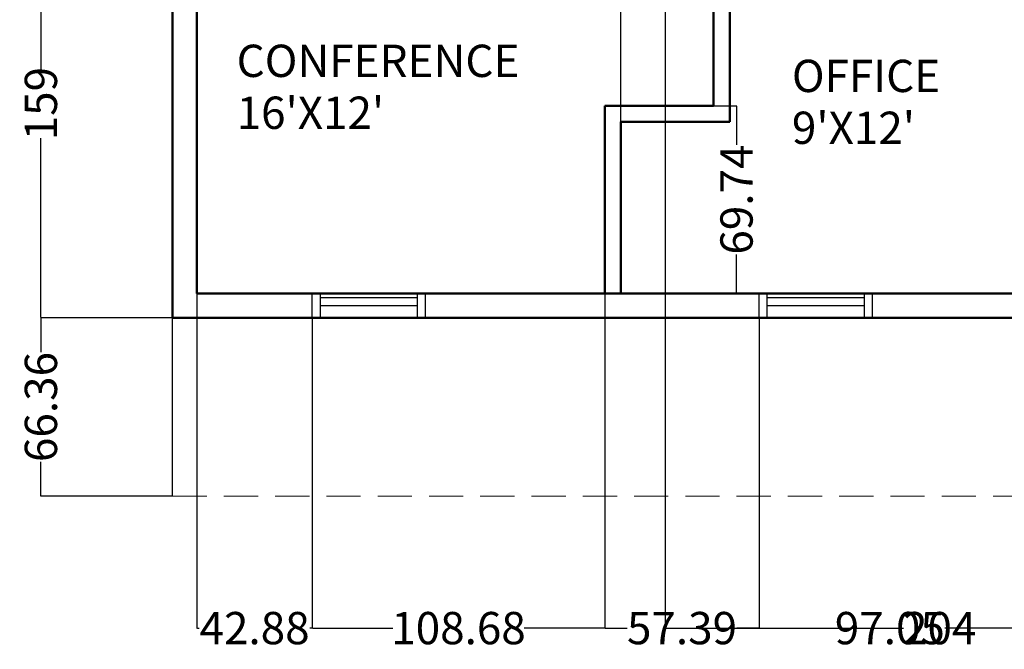
# Model space of a CAD drawing. Units: inches. Extents: x 128 to 1267, y -109 to 1208.
# Tile 5 of 8: x 180 to 546, y 608 to 842. Entities that reach past the tile are written whole.
import ezdxf

# ---------------------------------------------------------------- set-up
doc = ezdxf.new("R2010")
doc.units = ezdxf.units.IN
doc.header["$MEASUREMENT"] = 0
doc.linetypes.add('DASHED', pattern=[19.05, 12.7, -6.35])
for name, color, linetype, lineweight in [('A-ANNO-DIMS', 2, 'Continuous', 18), ('A-AREA-IDEN', 3, 'Continuous', 25), ('A-GLAZ', 3, 'Continuous', 25), ('A-ROOF-OVHD', 9, 'DASHED', 18), ('A-WALL', 7, 'Continuous', 50)]:
    doc.layers.add(name, color=color, linetype=linetype, lineweight=lineweight)
doc.styles.get("Standard").update_dxf_attribs({"font": 'arial.ttf'})
doc.dimstyles.get("Standard").update_dxf_attribs({"dimtxt": 12, "dimasz": 0.18, "dimexe": 0.18, "dimexo": 0.0625, "dimgap": 0.09, "dimtad": 0, "dimdec": 1, "dimzin": 0, "dimdsep": 46, "dimlunit": 3, "dimtxsty": 'Standard', "dimcen": 0.09, "dimadec": 0, "dimazin": 0, "dimtfac": 1, "dimtdec": 1, "dimtofl": 0, "dimtmove": 0, "dimatfit": 3, "dimfxl": 1, "dimtolj": 1, "dimtzin": 0, "dimarcsym": 0})

# ---------------------------------------------------------------- blocks, each defined once
blk = doc.blocks.new('WIN-900')
for p, q in [((1102.06, 345.56), (1111.06, 345.56)), ((1102.06, 342.56), (1111.06, 342.56)), ((1103.56, 306.56), (1103.56, 342.56)), ((1106.56, 306.56), (1106.56, 342.56)), ((1111.06, 306.56), (1102.06, 306.56)), ((1111.06, 303.56), (1102.06, 303.56))]:
    blk.add_line(p, q)
blk = doc.blocks.new('*D93')
at = {"layer": 'A-ANNO-DIMS', "color": 0, "lineweight": -2, "transparency": 16777216}
for p, q in [((237.13, 664.93), (237.13, 1188.36)), ((237.31, 1188.18), (667.76, 1188.18)), ((1124.95, 1188.18), (694.49, 1188.18)), ((1125.13, 664.93), (1125.13, 1188.36))]:
    blk.add_line(p, q, dxfattribs=at)
at = {"layer": 'A-ANNO-DIMS', "color": 0, "transparency": 16777216}
for points in [[(237.31, 1188.21), (237.31, 1188.15), (237.13, 1188.18)], [(1124.95, 1188.21), (1124.95, 1188.15), (1125.13, 1188.18)]]:
    blk.add_solid(points, dxfattribs=at)
at = {"layer": 'Defpoints', "color": 0, "transparency": 16777216}
for p in [(1125.13, 1188.18), (237.13, 664.87), (1125.13, 664.87)]:
    blk.add_point(p, dxfattribs=at)
at = {"layer": 'A-ANNO-DIMS', "color": 0, "transparency": 16777216, "insert": (681.13, 1188.18), "char_height": 12, "attachment_point": 5}
blk.add_mtext('\\A1;888', dxfattribs=at)
blk = doc.blocks.new('*D96')
at = {"layer": 'A-ANNO-DIMS', "color": 0, "lineweight": -2, "transparency": 16777216}
for p, q in [((237.06, 731.23), (188, 731.23)), ((188.18, 731.05), (188.18, 718.41)), ((188.18, 665.05), (188.18, 677.68)), ((237.06, 664.87), (188, 664.87))]:
    blk.add_line(p, q, dxfattribs=at)
at = {"layer": 'A-ANNO-DIMS', "color": 0, "transparency": 16777216}
for points in [[(188.15, 731.05), (188.21, 731.05), (188.18, 731.23)], [(188.15, 665.05), (188.21, 665.05), (188.18, 664.87)]]:
    blk.add_solid(points, dxfattribs=at)
at = {"layer": 'Defpoints', "color": 0, "transparency": 16777216}
for p in [(237.13, 731.23), (188.18, 664.87), (237.13, 664.87)]:
    blk.add_point(p, dxfattribs=at)
at = {"layer": 'A-ANNO-DIMS', "color": 0, "transparency": 16777216, "insert": (188.18, 698.05), "char_height": 12, "attachment_point": 5, "rotation": 90}
blk.add_mtext('\\A1;66.36', dxfattribs=at)
blk = doc.blocks.new('*D112')
at = {"layer": 'A-ANNO-DIMS', "color": 0, "lineweight": -2, "transparency": 16777216}
for p, q in [((246.13, 740.16), (246.13, 615.74)), ((289.01, 731.16), (289.01, 615.74)), ((246.31, 615.92), (246.98, 615.92)), ((288.83, 615.92), (288.16, 615.92))]:
    blk.add_line(p, q, dxfattribs=at)
at = {"layer": 'A-ANNO-DIMS', "color": 0, "transparency": 16777216}
for points in [[(246.31, 615.95), (246.31, 615.89), (246.13, 615.92)], [(288.83, 615.95), (288.83, 615.89), (289.01, 615.92)]]:
    blk.add_solid(points, dxfattribs=at)
at = {"layer": 'Defpoints', "color": 0, "transparency": 16777216}
for p in [(246.13, 740.23), (289.01, 731.23), (289.01, 615.92)]:
    blk.add_point(p, dxfattribs=at)
at = {"layer": 'A-ANNO-DIMS', "color": 0, "transparency": 16777216, "insert": (267.57, 615.92), "char_height": 12, "attachment_point": 5}
blk.add_mtext('\\A1;42.88', dxfattribs=at)
blk = doc.blocks.new('*D113')
at = {"layer": 'A-ANNO-DIMS', "color": 0, "lineweight": -2, "transparency": 16777216}
for p, q in [((397.68, 740.16), (397.68, 615.74)), ((289.01, 731.16), (289.01, 615.74)), ((289.19, 615.92), (318.9, 615.92)), ((397.5, 615.92), (367.79, 615.92))]:
    blk.add_line(p, q, dxfattribs=at)
at = {"layer": 'A-ANNO-DIMS', "color": 0, "transparency": 16777216}
for points in [[(289.19, 615.95), (289.19, 615.89), (289.01, 615.92)], [(397.5, 615.95), (397.5, 615.89), (397.68, 615.92)]]:
    blk.add_solid(points, dxfattribs=at)
at = {"layer": 'Defpoints', "color": 0, "transparency": 16777216}
for p in [(397.68, 740.23), (289.01, 731.23), (397.68, 615.92)]:
    blk.add_point(p, dxfattribs=at)
at = {"layer": 'A-ANNO-DIMS', "color": 0, "transparency": 16777216, "insert": (343.34, 615.92), "char_height": 12, "attachment_point": 5}
blk.add_mtext('\\A1;108.68', dxfattribs=at)
blk = doc.blocks.new('*D114')
at = {"layer": 'A-ANNO-DIMS', "color": 0, "lineweight": -2, "transparency": 16777216}
for p, q in [((397.68, 740.16), (397.68, 615.74)), ((455.08, 731.16), (455.08, 615.74)), ((397.86, 615.92), (406.03, 615.92)), ((454.9, 615.92), (446.73, 615.92))]:
    blk.add_line(p, q, dxfattribs=at)
at = {"layer": 'A-ANNO-DIMS', "color": 0, "transparency": 16777216}
for points in [[(397.86, 615.95), (397.86, 615.89), (397.68, 615.92)], [(454.9, 615.95), (454.9, 615.89), (455.08, 615.92)]]:
    blk.add_solid(points, dxfattribs=at)
at = {"layer": 'Defpoints', "color": 0, "transparency": 16777216}
for p in [(397.68, 740.23), (455.08, 731.23), (455.08, 615.92)]:
    blk.add_point(p, dxfattribs=at)
at = {"layer": 'A-ANNO-DIMS', "color": 0, "transparency": 16777216, "insert": (426.38, 615.92), "char_height": 12, "attachment_point": 5}
blk.add_mtext('\\A1;57.39', dxfattribs=at)
blk = doc.blocks.new('*D115')
at = {"layer": 'A-ANNO-DIMS', "color": 0, "lineweight": -2, "transparency": 16777216}
for p, q in [((552.13, 740.16), (552.13, 615.74)), ((455.08, 731.16), (455.08, 615.74)), ((455.26, 615.92), (483.22, 615.92)), ((551.95, 615.92), (523.98, 615.92))]:
    blk.add_line(p, q, dxfattribs=at)
at = {"layer": 'A-ANNO-DIMS', "color": 0, "transparency": 16777216}
for points in [[(455.26, 615.95), (455.26, 615.89), (455.08, 615.92)], [(551.95, 615.95), (551.95, 615.89), (552.13, 615.92)]]:
    blk.add_solid(points, dxfattribs=at)
at = {"layer": 'Defpoints', "color": 0, "transparency": 16777216}
for p in [(552.13, 740.23), (455.08, 731.23), (552.13, 615.92)]:
    blk.add_point(p, dxfattribs=at)
at = {"layer": 'A-ANNO-DIMS', "color": 0, "transparency": 16777216, "insert": (503.6, 615.92), "char_height": 12, "attachment_point": 5}
blk.add_mtext('\\A1;97.05', dxfattribs=at)
blk = doc.blocks.new('*D126')
at = {"layer": 'A-ANNO-DIMS', "color": 0, "lineweight": -2, "transparency": 16777216}
for p, q in [((246.06, 890.23), (188, 890.23)), ((188.18, 890.05), (188.18, 823.52)), ((188.18, 731.41), (188.18, 797.93)), ((237.06, 731.23), (188, 731.23))]:
    blk.add_line(p, q, dxfattribs=at)
at = {"layer": 'A-ANNO-DIMS', "color": 0, "transparency": 16777216}
for points in [[(188.15, 890.05), (188.21, 890.05), (188.18, 890.23)], [(188.15, 731.41), (188.21, 731.41), (188.18, 731.23)]]:
    blk.add_solid(points, dxfattribs=at)
at = {"layer": 'Defpoints', "color": 0, "transparency": 16777216}
for p in [(188.18, 890.23), (246.13, 890.23), (237.13, 731.23)]:
    blk.add_point(p, dxfattribs=at)
at = {"layer": 'A-ANNO-DIMS', "color": 0, "transparency": 16777216, "insert": (188.18, 810.73), "char_height": 12, "attachment_point": 5, "rotation": 90}
blk.add_mtext('\\A1;159', dxfattribs=at)
blk = doc.blocks.new('*D140')
at = {"layer": 'A-ANNO-DIMS', "color": 0, "lineweight": -2, "transparency": 16777216}
for p, q in [((397.74, 809.97), (446.81, 809.97)), ((446.63, 809.79), (446.63, 795.44)), ((446.63, 740.41), (446.63, 754.75)), ((397.74, 740.23), (446.81, 740.23))]:
    blk.add_line(p, q, dxfattribs=at)
at = {"layer": 'A-ANNO-DIMS', "color": 0, "transparency": 16777216}
for points in [[(446.6, 809.79), (446.66, 809.79), (446.63, 809.97)], [(446.6, 740.41), (446.66, 740.41), (446.63, 740.23)]]:
    blk.add_solid(points, dxfattribs=at)
at = {"layer": 'Defpoints', "color": 0, "transparency": 16777216}
for p in [(397.68, 809.97), (397.68, 740.23), (446.63, 740.23)]:
    blk.add_point(p, dxfattribs=at)
at = {"layer": 'A-ANNO-DIMS', "color": 0, "transparency": 16777216, "insert": (446.63, 775.1), "char_height": 12, "attachment_point": 5, "rotation": 90}
blk.add_mtext('\\A1;69.74', dxfattribs=at)
blk = doc.blocks.new('*D141')
at = {"layer": 'A-ANNO-DIMS', "color": 0, "lineweight": -2, "transparency": 16777216}
for p, q in [((403.68, 804.03), (403.68, 853.1)), ((403.86, 852.92), (443.95, 852.92)), ((444.13, 804.03), (444.13, 853.1)), ((444.13, 852.92), (444.31, 852.92))]:
    blk.add_line(p, q, dxfattribs=at)
at = {"layer": 'A-ANNO-DIMS', "color": 0, "transparency": 16777216}
for points in [[(403.86, 852.95), (403.86, 852.89), (403.68, 852.92)], [(443.95, 852.95), (443.95, 852.89), (444.13, 852.92)]]:
    blk.add_solid(points, dxfattribs=at)
at = {"layer": 'Defpoints', "color": 0, "transparency": 16777216}
for p in [(444.13, 852.92), (403.68, 803.97), (444.13, 803.97)]:
    blk.add_point(p, dxfattribs=at)
at = {"layer": 'A-ANNO-DIMS', "color": 0, "transparency": 16777216, "insert": (469.59, 852.92), "char_height": 12, "attachment_point": 5}
blk.add_mtext('\\A1;40.445', dxfattribs=at)
blk = doc.blocks.new('*D148')
at = {"layer": 'A-ANNO-DIMS', "color": 0, "lineweight": -2, "transparency": 16777216}
for p, q in [((420.13, 968.16), (420.13, 615.74)), ((624.13, 968.16), (624.13, 615.74)), ((420.31, 615.92), (508.7, 615.92)), ((623.95, 615.92), (535.55, 615.92))]:
    blk.add_line(p, q, dxfattribs=at)
at = {"layer": 'A-ANNO-DIMS', "color": 0, "transparency": 16777216}
for points in [[(420.31, 615.95), (420.31, 615.89), (420.13, 615.92)], [(623.95, 615.95), (623.95, 615.89), (624.13, 615.92)]]:
    blk.add_solid(points, dxfattribs=at)
at = {"layer": 'Defpoints', "color": 0, "transparency": 16777216}
for p in [(420.13, 968.23), (624.13, 968.23), (624.13, 615.92)]:
    blk.add_point(p, dxfattribs=at)
at = {"layer": 'A-ANNO-DIMS', "color": 0, "transparency": 16777216, "insert": (522.13, 615.92), "char_height": 12, "attachment_point": 5}
blk.add_mtext('\\A1;204', dxfattribs=at)

msp = doc.modelspace()

# ---------------------------------------------------------------- linework, layer by layer
at = {"layer": 'A-ROOF-OVHD'}
for p, q in [((237.1268, 731.2265), (237.1268, 664.8687)), ((237.1268, 664.8687), (1125.1268, 664.8687))]:
    msp.add_line(p, q, dxfattribs=at)
at = {"layer": 'A-WALL'}
for p, q in [((246.1268, 884.2265), (246.1268, 740.2265)), ((438.1268, 884.2265), (438.1268, 809.9714)), ((444.1268, 884.2265), (444.1268, 803.9714)), ((438.1268, 809.9714), (397.6821, 809.9714)), ((397.6821, 809.9714), (397.6821, 740.2265)), ((438.1268, 803.9714), (403.6821, 803.9714)), ((403.6821, 803.9714), (403.6821, 740.2265)), ((444.1268, 803.9714), (438.1268, 803.9714)), ((246.1268, 740.2265), (552.1268, 740.2265)), ((444.1268, 740.2265), (552.1268, 740.2265)), ((444.1268, 740.2265), (552.1268, 740.2265))]:
    msp.add_line(p, q, dxfattribs=at)
msp.add_lwpolyline([(1110.1268, 731.2265), (1125.1268, 731.2265), (1125.1268, 1139.2265), (237.1268, 1139.2265), (237.1268, 731.2265), (1038.1268, 731.2265)], dxfattribs=at)

# ---------------------------------------------------------------- block references
at = {"layer": 'A-GLAZ'}
for p, rotation in [((-14.5573, 1842.2825), 270.0000000000003), ((151.514, 1842.2825), 270.0000000000002)]:
    msp.add_blockref('WIN-900', p, dxfattribs=dict(at, rotation=rotation))

# ---------------------------------------------------------------- texts
at = {"layer": 'A-AREA-IDEN'}
for s, p in [('CONFERENCE', (260.9026, 820.6402)), ('OFFICE', (467.2124, 815.0458)), ("16'X12'", (260.9026, 801.3632)), ("9'X12'", (467.2124, 795.7689))]:
    msp.add_text(s, height=12, dxfattribs=at).set_placement(p)

# ---------------------------------------------------------------- dimensions: what is measured, and where the dimension line sits
at = {"layer": 'A-ANNO-DIMS'}
for base, p1, p2, override, picture, middle in [((1125.1268, 1188.1765), (237.1268, 664.8687), (1125.1268, 664.8687), {"dimdec": 0, "dimlfac": 1, "dimrnd": 0, "dimzin": 0, "dimdsep": 46, "dimlunit": 2}, '*D93', (681.1268, 1188.1765)), ((624.1268, 615.9187), (420.1268, 968.2265), (624.1268, 968.2265), {"dimdec": 0, "dimlfac": 1, "dimrnd": 0, "dimzin": 0, "dimdsep": 46, "dimlunit": 2}, '*D148', (522.1268, 615.9187)), ((444.1268, 852.9214), (403.6821, 803.9714), (444.1268, 803.9714), {"dimdec": 3, "dimlfac": 1, "dimrnd": 0, "dimzin": 0, "dimdsep": 46, "dimlunit": 2}, '*D141', (469.5919, 852.9214)), ((289.005, 615.9187), (246.1268, 740.2265), (289.005, 731.2265), {"dimdec": 2, "dimlfac": 1, "dimrnd": 0, "dimzin": 0, "dimdsep": 46, "dimlunit": 2}, '*D112', (267.5659, 615.9187)), ((397.6821, 615.9187), (289.005, 731.2265), (397.6821, 740.2265), {"dimdec": 2, "dimlfac": 1, "dimrnd": 0, "dimzin": 0, "dimdsep": 46, "dimlunit": 2}, '*D113', (343.3435, 615.9187)), ((455.0763, 615.9187), (397.6821, 740.2265), (455.0763, 731.2265), {"dimdec": 2, "dimlfac": 1, "dimrnd": 0, "dimzin": 0, "dimdsep": 46, "dimlunit": 2}, '*D114', (426.3792, 615.9187)), ((552.1268, 615.9187), (455.0763, 731.2265), (552.1268, 740.2265), {"dimdec": 2, "dimlfac": 1, "dimrnd": 0, "dimzin": 0, "dimdsep": 46, "dimlunit": 2}, '*D115', (503.6015, 615.9187))]:
    dim = msp.add_linear_dim(base=base, p1=p1, p2=p2, dimstyle='Standard', override=override, dxfattribs=at)
    dim.commit()
    dim.dimension.update_dxf_attribs({"geometry": picture, "text_midpoint": middle})
for base, p1, p2, angle, override, picture, middle in [((188.1768, 890.2265), (237.1268, 731.2265), (246.1268, 890.2265), 90, {"dimdec": 0, "dimlfac": 1, "dimrnd": 0, "dimzin": 0, "dimdsep": 46, "dimlunit": 2}, '*D126', (188.1768, 810.7265)), ((446.6321, 740.2265), (397.6821, 809.9714), (397.6821, 740.2265), 270, {"dimdec": 2, "dimlfac": 1, "dimrnd": 0, "dimzin": 0, "dimdsep": 46, "dimlunit": 2}, '*D140', (446.6321, 775.0989)), ((188.1768, 664.8687), (237.1268, 731.2265), (237.1268, 664.8687), 90, {"dimdec": 2, "dimlfac": 1, "dimrnd": 0, "dimzin": 0, "dimdsep": 46, "dimlunit": 2}, '*D96', (188.1768, 698.0476))]:
    dim = msp.add_linear_dim(base=base, p1=p1, p2=p2, angle=angle, dimstyle='Standard', override=override, dxfattribs=at)
    dim.commit()
    dim.dimension.update_dxf_attribs({"geometry": picture, "text_midpoint": middle})

doc.saveas('drawing.dxf')
